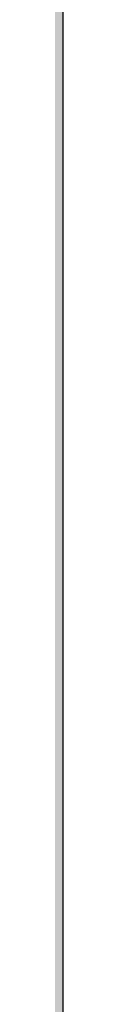
# Model space of a CAD drawing. Units: inches. Extents: x 2091 to 2899, y 967 to 2217.
# Tile 63 of 256: x 2212.1436 to 2212.1443, y 1100.1654 to 1100.4988. Entities that reach past the tile are written whole.
import ezdxf

# ---------------------------------------------------------------- set-up
doc = ezdxf.new("R2010")
doc.units = ezdxf.units.IN
doc.layers.add('A-ANNO-DIMS', color=2, linetype='Continuous', lineweight=18)
doc.layers.add('A-WALL-PATT', color=141, linetype='Continuous', lineweight=13, true_color=0xadddf7)
doc.styles.get("Standard").update_dxf_attribs({"font": 'arial.ttf'})
doc.dimstyles.new('ISO-25', dxfattribs={"dimtxt": 4, "dimasz": 4, "dimexe": 1.25, "dimexo": 0.625, "dimtad": 1, "dimdec": 0, "dimlunit": 3, "dimtxsty": 'Standard', "dimcen": 2.5, "dimadec": 0, "dimazin": 0, "dimtfac": 1, "dimtdec": 0, "dimtmove": 0, "dimatfit": 3, "dimfxl": 1, "dimarcsym": 0})

# ---------------------------------------------------------------- blocks, each defined once
blk = doc.blocks.new('*D71')
at = {"layer": 'A-ANNO-DIMS', "color": 0, "lineweight": -2, "transparency": 16777216}
for p, q in [((2212.1436, 1351.29406), (2212.1436, 969.4643)), ((2452.1436, 1351.29406), (2452.1436, 969.4643)), ((2216.1436, 970.7143), (2448.1436, 970.7143))]:
    blk.add_line(p, q, dxfattribs=at)
at = {"layer": 'A-ANNO-DIMS', "color": 0, "transparency": 16777216}
for points in [[(2216.1436, 971.38097), (2216.1436, 970.04764), (2212.1436, 970.7143)], [(2448.1436, 971.38097), (2448.1436, 970.04764), (2452.1436, 970.7143)]]:
    blk.add_solid(points, dxfattribs=at)
at = {"layer": 'Defpoints', "color": 0, "transparency": 16777216}
for p in [(2212.1436, 1351.91906), (2452.1436, 1351.91906), (2452.1436, 970.7143)]:
    blk.add_point(p, dxfattribs=at)
at = {"layer": 'A-ANNO-DIMS', "color": 0, "transparency": 16777216, "insert": (2332.1436, 973.38159), "char_height": 4, "attachment_point": 5}
blk.add_mtext('20\'-0"', dxfattribs=at)
blk = doc.blocks.new('*D75')
at = {"layer": 'A-ANNO-DIMS', "color": 0, "lineweight": -2, "transparency": 16777216}
for p, q in [((2212.1436, 1274.79406), (2212.1436, 969.4643)), ((2308.1436, 1274.79406), (2308.1436, 969.4643)), ((2216.1436, 970.7143), (2304.1436, 970.7143))]:
    blk.add_line(p, q, dxfattribs=at)
at = {"layer": 'A-ANNO-DIMS', "color": 0, "transparency": 16777216}
for points in [[(2216.1436, 971.38097), (2216.1436, 970.04764), (2212.1436, 970.7143)], [(2304.1436, 971.38097), (2304.1436, 970.04764), (2308.1436, 970.7143)]]:
    blk.add_solid(points, dxfattribs=at)
at = {"layer": 'Defpoints', "color": 0, "transparency": 16777216}
for p in [(2212.1436, 1275.41906), (2308.1436, 1275.41906), (2308.1436, 970.7143)]:
    blk.add_point(p, dxfattribs=at)
at = {"layer": 'A-ANNO-DIMS', "color": 0, "transparency": 16777216, "insert": (2260.1436, 973.38159), "char_height": 4, "attachment_point": 5}
blk.add_mtext('8\'-0"', dxfattribs=at)
blk = doc.blocks.new('*D91')
at = {"layer": 'A-ANNO-DIMS', "color": 0, "lineweight": -2, "transparency": 16777216}
for p, q in [((2211.65063, 1152.24706), (2098.31133, 1152.24706)), ((2099.56133, 1103.91906), (2099.56133, 1148.24706)), ((2211.5186, 1099.91906), (2098.31133, 1099.91906))]:
    blk.add_line(p, q, dxfattribs=at)
at = {"layer": 'A-ANNO-DIMS', "color": 0, "transparency": 16777216}
for points in [[(2098.89467, 1148.24706), (2100.228, 1148.24706), (2099.56133, 1152.24706)], [(2098.89467, 1103.91906), (2100.228, 1103.91906), (2099.56133, 1099.91906)]]:
    blk.add_solid(points, dxfattribs=at)
at = {"layer": 'Defpoints', "color": 0, "transparency": 16777216}
for p in [(2099.56133, 1152.24706), (2212.27563, 1152.24706), (2212.1436, 1099.91906)]:
    blk.add_point(p, dxfattribs=at)
at = {"layer": 'A-ANNO-DIMS', "color": 0, "transparency": 16777216, "insert": (2096.86812, 1126.08306), "char_height": 4, "attachment_point": 5, "rotation": 90}
blk.add_mtext('4\'-4 1/2"', dxfattribs=at)

msp = doc.modelspace()

# ---------------------------------------------------------------- hatches: boundary and pattern name
at = {"layer": 'A-WALL-PATT'}
h = msp.add_hatch(color=256, dxfattribs=at)
h.dxf.hatch_style = 1
h.paths.add_polyline_path([(2803.1436, 2050.91906), (2203.1436, 2050.91906), (2203.1436, 1090.91906), (2803.1436, 1090.91906)])
h.paths.add_polyline_path([(2635.79885, 1147.54046), (2674.52405, 1147.54046, 0.376086), (2678.52967, 1152.8802), (2678.52967, 1159.55647, 0.333335), (2674.52432, 1163.56185), (2674.52432, 1163.56185), (2674.52432, 1192.93439), (2635.80597, 1192.93439), (2597.08762, 1192.93439), (2597.08762, 1163.56185, 0.333335), (2593.08228, 1159.55647), (2593.08228, 1152.8802, 0.376086), (2597.08789, 1147.54046)], flags=0)
h.paths.add_polyline_path([(2436.01043, 1278.24078, 0.000483), (2435.95264, 1278.21503, -0.001328), (2435.93563, 1278.11169, -0.001711), (2436.11644, 1278.04076, 0.002185)], flags=0)
h.paths.add_polyline_path([(2794.1436, 1143.41906), (2794.1436, 1347.41906), (2543.37017, 1347.41906), (2543.37017, 1351.91906), (2794.1436, 1351.91906), (2794.1436, 1392.71355), (2793.9474, 1392.71355), (2793.9474, 1473.5369), (2794.1436, 1473.5369), (2794.1436, 1531.91906), (2650.1436, 1531.91906), (2650.1436, 1536.41906), (2794.1436, 1536.41906), (2794.1436, 1692.41906), (2609.37561, 1692.41906), (2609.37561, 1644.41906), (2604.87561, 1644.41906), (2604.87561, 1744.91906), (2609.37561, 1744.91906), (2609.37561, 1696.91906), (2794.1436, 1696.91906), (2794.1436, 1780.91906), (2609.6436, 1780.91906), (2493.87561, 1780.91906), (2493.87561, 1785.41906), (2609.6436, 1785.41906), (2794.1436, 1785.41906), (2794.1436, 1847.93882), (2793.95122, 1847.93882), (2793.95122, 1928.76217), (2794.1436, 1928.76217), (2794.1436, 1941.41906), (2614.1436, 1941.41906), (2614.1436, 1821.41906), (2609.6436, 1821.41906), (2609.6436, 1941.41906), (2392.1436, 1941.41906), (2392.1436, 1819.91906), (2387.6436, 1819.91906), (2387.6436, 1941.41906), (2212.1436, 1941.41906), (2212.1436, 1783.91906), (2392.1436, 1783.91906), (2392.1436, 1780.91906), (2212.1436, 1780.91906), (2212.1436, 1629.41906), (2387.6436, 1629.41906), (2387.6436, 1744.91906), (2392.1436, 1744.91906), (2392.1436, 1627.91906), (2317.1436, 1627.91906), (2317.1436, 1551.41906), (2317.1436, 1536.41906), (2459.38359, 1536.41906), (2459.38359, 1602.39648), (2463.88359, 1602.39648), (2463.88359, 1531.91906), (2456.6436, 1531.91906), (2456.6436, 1529.91906), (2452.1436, 1529.91906), (2452.1436, 1531.91906), (2312.6436, 1531.91906), (2312.6436, 1551.41906), (2306.1436, 1551.41906), (2306.1436, 1555.91906), (2308.1436, 1555.91906), (2308.1436, 1551.41906), (2312.6436, 1551.41906), (2312.6436, 1627.91906), (2212.1436, 1627.91906), (2212.1436, 1555.91906), (2270.1436, 1555.91906), (2270.1436, 1551.41906), (2212.1436, 1551.41906), (2212.1436, 1351.91906), (2272.1436, 1351.91906), (2272.1436, 1347.41906), (2212.1436, 1347.41906), (2212.1436, 1275.41906), (2308.1436, 1275.41906), (2308.1436, 1351.91906), (2452.1436, 1351.91906), (2452.1436, 1493.91906), (2456.6436, 1493.91906), (2456.6436, 1347.41906), (2312.6436, 1347.41906), (2312.6436, 1270.91906), (2212.1436, 1270.91906), (2212.1436, 1099.91906), (2281.23752, 1099.91906), (2282.87104, 1110.9138), (2282.00834, 1116.9966), (2278.55774, 1121.4204), (2268.20564, 1128.0562), (2272.08764, 1128.0562), (2273.81294, 1131.927), (2279.42034, 1134.6919), (2285.02784, 1135.2449), (2287.61584, 1137.4568), (2288.04714, 1138.0098), (2289.34114, 1140.7747), (2291.06654, 1139.6687), (2292.36054, 1135.2449), (2295.37984, 1136.9038), (2296.24254, 1135.7979), (2297.10524, 1133.033), (2300.12464, 1138.0098), (2303.14394, 1138.0098), (2304.43794, 1135.7979), (2303.14394, 1133.586), (2306.59464, 1134.6919), (2307.88874, 1133.033), (2310.90804, 1135.2449), (2313.92744, 1134.1389), (2315.62686, 1132.4271), (2308.32004, 1117.5496), (2290.20384, 1109.8079), (2288.90984, 1103.1721), (2289.27231, 1099.91906), (2434.91823, 1099.91906), (2431.59323, 1124.78806), (2429.93023, 1169.55306), (2430.92718, 1240.51969), (2435.65893, 1238.18613), (2437.13523, 1196.55406), (2438.79823, 1143.97306), (2442.67823, 1111.99806), (2446.55823, 1099.91906), (2794.1436, 1099.91906), (2794.1436, 1138.91906), (2548.03245, 1138.91906), (2548.03245, 1143.41906), (2548.03245, 1148.81906), (2546.66846, 1148.03156), (2528.68569, 1179.17862, 0.256256), (2512.03245, 1148.81906), (2512.03245, 1143.41906), (2512.03245, 1138.91906), (2507.53245, 1138.91906), (2507.53245, 1143.41906), (2507.53245, 1148.81906, 0.256256), (2490.8792, 1179.17862), (2472.89644, 1148.03156), (2471.53245, 1148.81906), (2471.53245, 1143.41906), (2467.03245, 1143.41906), (2467.03245, 1269.94579, 0.039061), (2460.90999, 1273.58006), (2467.03245, 1273.58006), (2467.03245, 1286.32536, 0.014511), (2465.21619, 1286.76191), (2467.03245, 1287.05258), (2467.03245, 1323.41906), (2471.53245, 1323.41906), (2471.53245, 1148.81906), (2489.53245, 1179.99597), (2490.89644, 1179.20847), (2490.8792, 1179.17862, -0.256256), (2507.53245, 1148.81906), (2507.53245, 1143.41906), (2512.03245, 1143.41906), (2512.03245, 1148.81906, -0.256256), (2528.68569, 1179.17862), (2528.66846, 1179.20847), (2530.03245, 1179.99597), (2548.03245, 1148.81906), (2548.03245, 1143.41906)], flags=16)
h.paths.add_polyline_path([(2607.76855, 1200.94508), (2607.76855, 1265.03063), (2597.08762, 1281.05201), (2619.78459, 1281.05201), (2627.79528, 1337.12686), (2635.79885, 1337.12686), (2643.81666, 1337.12686), (2651.82736, 1281.05201), (2674.52432, 1281.05201), (2663.8434, 1265.03063), (2663.8434, 1200.94508), (2635.80597, 1200.94508)], flags=0)
edge = h.paths.add_edge_path(flags=0)
edge.add_ellipse((13303.89622, 1272.99872), major_axis=(-10595.31304, 0), ratio=0.84230387009, start_angle=0.628237219, end_angle=0.6465541, ccw=False)
edge.add_ellipse((2711.70045, 1156.85268), major_axis=(2.21977, 0), ratio=0.8423039, start_angle=111.53524, end_angle=180.62824, ccw=False)
edge.add_ellipse((13303.15629, 1272.99872), major_axis=(-10593.02631, 0), ratio=0.84230386954, start_angle=0.528271472, end_angle=0.646554097, ccw=False)
edge.add_line((2710.7646, 1175.3333), (2710.12999, 1175.3333))
edge.add_ellipse((2710.12999, 1176.57978), major_axis=(1.47985, 0), ratio=0.8423039, start_angle=180, end_angle=270, ccw=False)
edge.add_line((2708.65014, 1176.57978), (2708.65014, 1200.78291))
edge.add_ellipse((2710.12999, 1200.78291), major_axis=(1.47985, 0), ratio=0.8423039, start_angle=90, end_angle=180, ccw=False)
edge.add_line((2710.12999, 1202.02939), (2710.46508, 1202.02939))
edge.add_ellipse((13303.15629, 1272.99872), major_axis=(-10593.02631, 0), ratio=0.84230386954, start_angle=-0.090229089, end_angle=0.383866779, ccw=False)
edge.add_ellipse((2710.12999, 1290.92703), major_axis=(-1.47985, 0), ratio=0.8423039, start_angle=0, end_angle=90, ccw=False)
edge.add_line((2708.65014, 1290.92703), (2708.65014, 1315.13017))
edge.add_ellipse((2710.12999, 1315.13017), major_axis=(-1.47985, 0), ratio=0.8423039, start_angle=-90, end_angle=0, ccw=False)
edge.add_line((2710.12999, 1316.37665), (2710.70631, 1316.37665))
edge.add_ellipse((3238.40172, 1296.28957), major_axis=(528.234, 0), ratio=0.84230387, start_angle=176.3495724, end_angle=177.8200497, ccw=False)
edge.add_ellipse((2775.06304, 1071.4507), major_axis=(313.30776, 0), ratio=0.84230387, start_angle=102.1259656, end_angle=103.780529, ccw=False)
edge.add_ellipse((2775.06304, 1078.3057), major_axis=(-305.30289, 0), ratio=0.84230387, start_angle=-79.790461, end_angle=-77.5553727, ccw=False)
edge.add_ellipse((2695.14177, 1541.97538), major_axis=(-250.96022, 0), ratio=0.84230387, start_angle=99.256566, end_angle=102.5549326)
edge.add_line((2741.41033, 1334.21426), (2747.13255, 1337.37848))
edge.add_ellipse((2747.53862, 1336.85748), major_axis=(-0.73992, 0), ratio=0.842304, start_angle=270, end_angle=307.93313, ccw=False)
edge.add_ellipse((2747.53862, 1336.85748), major_axis=(-0.73992, 0), ratio=0.842304, start_angle=232.06687, end_angle=270, ccw=False)
edge.add_line((2747.94469, 1337.37848), (2753.66691, 1334.21426))
edge.add_ellipse((2799.93547, 1541.97538), major_axis=(250.96022, 0), ratio=0.84230387, start_angle=257.4450674, end_angle=260.743434)
edge.add_ellipse((2720.01419, 1078.3057), major_axis=(305.30289, 0), ratio=0.84230387, start_angle=77.5553727, end_angle=79.790461, ccw=False)
edge.add_ellipse((2720.01419, 1071.4507), major_axis=(-313.30776, 0), ratio=0.84230387, start_angle=256.219471, end_angle=257.8740344, ccw=False)
edge.add_ellipse((2256.67551, 1296.28957), major_axis=(-528.234, 0), ratio=0.84230387, start_angle=182.1799503, end_angle=183.6504276, ccw=False)
edge.add_line((2784.37092, 1316.37665), (2784.94725, 1316.37665))
edge.add_ellipse((2784.94725, 1315.13017), major_axis=(1.47985, 0), ratio=0.8423039, start_angle=0, end_angle=90, ccw=False)
edge.add_line((2786.42709, 1315.13017), (2786.42709, 1290.92703))
edge.add_ellipse((2784.94725, 1290.92703), major_axis=(1.47985, 0), ratio=0.8423039, start_angle=270, end_angle=360, ccw=False)
edge.add_ellipse((-7808.07906, 1272.99872), major_axis=(10593.02631, 0), ratio=0.84230386954, start_angle=-0.383866779, end_angle=0.090229089, ccw=False)
edge.add_line((2784.61216, 1202.02939), (2784.94725, 1202.02939))
edge.add_ellipse((2784.94725, 1200.78291), major_axis=(1.47985, 0), ratio=0.8423039, start_angle=0, end_angle=90, ccw=False)
edge.add_line((2786.42709, 1200.78291), (2786.42709, 1176.57978))
edge.add_ellipse((2784.94725, 1176.57978), major_axis=(-1.47985, 0), ratio=0.8423039, start_angle=90, end_angle=180, ccw=False)
edge.add_line((2784.94725, 1175.3333), (2784.31264, 1175.3333))
edge.add_ellipse((-7808.07906, 1272.99872), major_axis=(10593.02631, 0), ratio=0.84230386954, start_angle=-0.618643196, end_angle=-0.528271472, ccw=False)
edge.add_ellipse((2783.37678, 1156.85268), major_axis=(-2.21977, 0), ratio=0.8423039, start_angle=179.37176, end_angle=248.46476, ccw=False)
edge.add_ellipse((-7808.81898, 1272.99872), major_axis=(-10595.31304, 0), ratio=0.84230386576, start_angle=179.353445923, end_angle=179.371762803, ccw=False)
edge.add_ellipse((2780.2973, 1153.50079), major_axis=(-5.24643, 0), ratio=0.8423039, start_angle=90, end_angle=179.35345, ccw=False)
edge.add_line((2780.2973, 1149.08171), (2714.77993, 1149.08171))
edge.add_ellipse((2714.77993, 1153.50079), major_axis=(5.24643, 0), ratio=0.8423039, start_angle=180.64655, end_angle=270, ccw=False)
edge = h.paths.add_edge_path(flags=0)
edge.add_line((2718.18737, 1151.00783), (2718.18737, 1170.47236))
edge.add_ellipse((2721.14706, 1170.47236), major_axis=(-2.95969, 0), ratio=0.8423039, start_angle=-90, end_angle=0, ccw=False)
edge.add_line((2721.14706, 1172.96532), (2773.93017, 1172.96532))
edge.add_ellipse((2773.93017, 1170.47236), major_axis=(-2.95969, 0), ratio=0.8423039, start_angle=180, end_angle=270, ccw=False)
edge.add_line((2776.88987, 1170.47236), (2776.88987, 1151.00783))
edge.add_line((2776.88987, 1151.00783), (2718.18737, 1151.00783))
edge = h.paths.add_edge_path(flags=0)
edge.add_line((2718.18737, 1180.23415), (2718.18737, 1199.05783))
edge.add_ellipse((2747.53862, 1320.39864), major_axis=(147.01792, 0), ratio=0.84230387, start_angle=256.4018653, end_angle=283.5981347)
edge.add_line((2776.88987, 1199.05783), (2776.88987, 1180.23415))
edge.add_ellipse((2747.53862, 1301.57496), major_axis=(147.01792, 0), ratio=0.84230387, start_angle=256.4018653, end_angle=283.5981347, ccw=False)
edge = h.paths.add_edge_path(flags=0)
edge.add_ellipse((13303.15629, 1272.99872), major_axis=(-10591.54646, 0), ratio=0.84230386955, start_angle=0.055594314, end_angle=0.377764194, ccw=False)
edge.add_line((2711.61686, 1262.72171), (2715.66741, 1249.4954))
edge.add_ellipse((6413.89196, 1241.69192), major_axis=(-3698.23616, 0), ratio=0.8423038695, start_angle=-0.12089737, end_angle=0.36407635)
edge.add_line((2715.76104, 1218.19245), (2711.93431, 1203.16736))
edge = h.paths.add_edge_path(flags=0)
edge.add_line((2718.18737, 1251.07457), (2716.00249, 1267.45044))
edge.add_ellipse((2742.15117, 1202.18954), major_axis=(81.77258, 0), ratio=0.84230387, start_angle=94.277421, end_angle=111.8349538, ccw=False)
edge.add_line((2737.00975, 1270.93063), (2758.06748, 1270.93063))
edge.add_ellipse((2752.92606, 1202.18954), major_axis=(81.77258, 0), ratio=0.84230387, start_angle=68.1650462, end_angle=85.722579, ccw=False)
edge.add_line((2779.07475, 1267.45044), (2776.88987, 1251.07457))
edge.add_ellipse((2750.33806, 1187.88536), major_axis=(79.57966, 0), ratio=0.84230387, start_angle=67.2080851, end_angle=85.1299304)
edge.add_line((2756.03466, 1254.74366), (2739.04258, 1254.74366))
edge.add_ellipse((2744.73917, 1187.88536), major_axis=(79.57966, 0), ratio=0.84230387, start_angle=94.8700696, end_angle=112.7919149)
edge = h.paths.add_edge_path(flags=0)
edge.add_line((2783.14293, 1203.16736), (2779.31619, 1218.19245))
edge.add_ellipse((-918.81473, 1241.69192), major_axis=(3698.23616, 0), ratio=0.8423038695, start_angle=-0.36407635, end_angle=0.12089737)
edge.add_line((2779.40983, 1249.4954), (2783.46037, 1262.72171))
edge.add_ellipse((-7808.07906, 1272.99872), major_axis=(-10591.54646, 0), ratio=0.84230386954, start_angle=179.622235806, end_angle=179.944405687, ccw=False)
edge = h.paths.add_edge_path(flags=0)
edge.add_ellipse((2734.20089, 1286.69044), major_axis=(-0.35661, 6.34008), ratio=0.6038336, start_angle=89.002014, end_angle=253.657408, ccw=False)
edge.add_line((2730.369, 1286.54181), (2730.369, 1301.35198))
edge.add_line((2730.369, 1301.35198), (2735.91331, 1305.2148))
edge.add_ellipse((2736.38492, 1304.73456), major_axis=(0.73992, 0), ratio=0.842304, start_angle=90, end_angle=134.48021, ccw=False)
edge.add_line((2736.38492, 1305.3578), (2738.03278, 1305.3578))
edge.add_line((2738.03278, 1305.3578), (2738.03278, 1307.70793))
edge.add_ellipse((2794.20164, 1307.70793), major_axis=(56.16886, 0), ratio=0.84230387, start_angle=150.56143, end_angle=180, ccw=False)
edge.add_ellipse((2700.87559, 1307.70793), major_axis=(-56.16886, 0), ratio=0.84230387, start_angle=180, end_angle=209.43857, ccw=False)
edge.add_line((2757.04445, 1307.70793), (2757.04445, 1305.3578))
edge.add_line((2757.04445, 1305.3578), (2758.69232, 1305.3578))
edge.add_ellipse((2758.69232, 1304.73456), major_axis=(-0.73992, 0), ratio=0.842304, start_angle=225.51979, end_angle=270, ccw=False)
edge.add_line((2759.16392, 1305.2148), (2764.70823, 1301.35198))
edge.add_line((2764.70823, 1301.35198), (2764.70823, 1286.54181))
edge.add_ellipse((2760.87634, 1286.69044), major_axis=(0.35661, 6.34008), ratio=0.6038336, start_angle=106.342592, end_angle=270.997986, ccw=False)
edge.add_line((2757.04445, 1285.79709), (2757.04445, 1307.70793))
edge.add_ellipse((2700.87559, 1307.70793), major_axis=(-56.16886, 0), ratio=0.84230387, start_angle=180, end_angle=209.43857)
edge.add_ellipse((2794.20164, 1307.70793), major_axis=(56.16886, 0), ratio=0.84230387, start_angle=150.56143, end_angle=180)
edge.add_line((2738.03278, 1307.70793), (2738.03278, 1285.79709))
h.paths.add_polyline_path([(2417.81227, 1104.4497), (2413.49227, 1102.5297), (2410.61227, 1103.9697), (2409.17227, 1106.3697), (2407.25227, 1107.3297), (2406.29227, 1109.7297), (2405.33227, 1114.0497), (2405.33227, 1117.8897), (2406.29227, 1120.1297), (2407.25227, 1119.8097), (2408.84832, 1118.32766), (2410.17395, 1119.42417), (2410.21127, 1120.4057), (2411.04073, 1121.41905), (2410.69927, 1119.8587), (2410.17395, 1119.42417), (2410.08845, 1117.17611), (2411.13284, 1116.20632), (2413.97227, 1119.3297), (2416.85227, 1120.7697), (2416.86972, 1120.79878), (2417.03507, 1119.40512), (2417.89621, 1118.14338), (2418.29227, 1118.3697), (2419.54445, 1120.03927), (2419.36092, 1118.38749), (2419.03211, 1119.35615), (2418.39894, 1118.51193), (2419.25227, 1114.5297), (2418.79409, 1107.19879)], flags=0)
h.paths.add_polyline_path([(2508.87017, 1347.41906), (2508.37017, 1347.41906), (2508.37017, 1351.91906), (2508.87017, 1351.91906)], flags=0)
h.paths.add_polyline_path([(2473.37017, 1347.41906), (2472.37017, 1347.41906), (2467.87017, 1347.41906), (2467.87017, 1455.41906), (2472.37017, 1455.41906), (2472.37017, 1352.41906), (2473.37017, 1352.41906)], flags=0)
h.paths.add_polyline_path([(2352.10624, 1217.4462), (2349.22624, 1218.8862), (2347.78624, 1221.2862), (2345.86624, 1222.2462), (2344.90624, 1224.6462), (2343.94624, 1228.9662), (2343.94624, 1232.8062), (2344.90624, 1235.0462), (2345.86624, 1234.7262), (2347.46229, 1233.24415), (2348.78792, 1234.34066), (2348.82524, 1235.3222), (2349.6547, 1236.33555), (2349.31324, 1234.7752), (2348.78792, 1234.34066), (2348.70242, 1232.0926), (2349.74681, 1231.12282), (2352.58624, 1234.2462), (2355.46624, 1235.6862), (2355.48369, 1235.71528), (2355.64904, 1234.32161), (2356.51018, 1233.05988), (2356.90624, 1233.2862), (2358.15842, 1234.95576), (2357.97489, 1233.30398), (2357.64608, 1234.27264), (2357.01291, 1233.42842), (2357.86624, 1229.4462), (2357.40806, 1222.11529), (2356.42624, 1219.3662)], flags=0)
h.paths.add_polyline_path([(2348.2968, 1112.22442), (2347.0138, 1112.31042), (2345.5298, 1114.12742), (2345.7318, 1115.85842), (2346.8118, 1116.98242), (2346.8118, 1114.64642), (2345.8668, 1114.21442), (2346.8798, 1114.30042)], flags=0)
h.paths.add_polyline_path([(2347.0138, 1110.92642), (2346.2718, 1110.49342), (2346.6098, 1111.18642)], flags=0)
h.paths.add_polyline_path([(2345.8668, 1118.19442), (2345.5298, 1117.32942), (2343.7078, 1118.02142), (2344.3828, 1118.62642)], flags=0)
h.paths.add_polyline_path([(2346.6768, 1109.28242), (2346.0698, 1108.07142), (2345.8668, 1110.06142)], flags=0)
h.paths.add_polyline_path([(2345.0568, 1119.75142), (2343.6398, 1119.75142), (2343.9778, 1121.13542)], flags=0)
h.paths.add_polyline_path([(2345.2598, 1116.55042), (2345.1248, 1115.85842), (2344.9218, 1115.68542), (2344.7198, 1116.37742)], flags=0)
h.paths.add_polyline_path([(2345.6648, 1112.31042), (2345.4618, 1111.53242), (2344.0448, 1111.96442), (2344.6518, 1112.57042)], flags=0)
h.paths.add_polyline_path([(2345.1918, 1113.34942), (2344.4498, 1113.86842), (2344.7198, 1114.38742)], flags=0)
h.paths.add_polyline_path([(2344.6518, 1116.80942), (2344.1798, 1115.68542), (2344.6518, 1115.33942), (2343.9098, 1114.90642), (2343.0328, 1115.94442), (2343.6398, 1116.46342)], flags=0)
h.paths.add_polyline_path([(2345.8668, 1106.68642), (2344.9898, 1105.56242), (2344.5168, 1106.60042)], flags=0)
h.paths.add_polyline_path([(2344.8548, 1110.06142), (2344.5168, 1109.28242), (2344.1128, 1109.71542)], flags=0)
h.paths.add_polyline_path([(2344.0448, 1113.52242), (2343.4378, 1113.08942), (2342.7628, 1113.95442)], flags=0)
h.paths.add_polyline_path([(2344.3148, 1111.01242), (2342.9648, 1110.32042), (2342.9648, 1111.09942)], flags=0)
h.paths.add_polyline_path([(2345.1248, 1104.69742), (2344.5848, 1103.74542), (2344.4498, 1104.26442)], flags=0)
h.paths.add_polyline_path([(2342.8298, 1121.22242), (2341.7498, 1120.53042), (2340.5358, 1121.04942), (2340.1308, 1121.82842), (2340.6708, 1122.95242), (2341.1428, 1121.82842), (2341.6148, 1122.00142)], flags=0)
h.paths.add_polyline_path([(2342.9648, 1119.75142), (2343.0328, 1118.45342), (2342.0878, 1118.02142), (2342.0198, 1119.49142)], flags=0)
h.paths.add_polyline_path([(2342.6948, 1116.89642), (2341.9528, 1116.63642), (2342.0198, 1117.32942)], flags=0)
h.paths.add_polyline_path([(2343.0328, 1112.22442), (2342.0198, 1111.79142), (2341.5478, 1112.22442), (2342.3578, 1113.34942)], flags=0)
h.paths.add_polyline_path([(2343.7748, 1104.43742), (2342.6278, 1102.88042), (2342.6948, 1104.61042), (2343.4378, 1105.12942)], flags=0)
h.paths.add_polyline_path([(2342.0198, 1115.07942), (2340.8058, 1115.51242), (2340.9408, 1116.37742)], flags=0)
h.paths.add_polyline_path([(2341.4808, 1120.09742), (2341.4808, 1119.40542), (2341.0758, 1119.57842), (2341.1428, 1120.09742)], flags=0)
h.paths.add_polyline_path([(2341.8178, 1114.47342), (2340.9408, 1113.08942), (2340.8058, 1114.56042)], flags=0)
h.paths.add_polyline_path([(2341.1428, 1118.54042), (2340.9408, 1116.98242), (2339.0508, 1117.67542), (2339.0508, 1118.62642)], flags=0)
h.paths.add_polyline_path([(2342.6948, 1101.66842), (2341.9528, 1101.84142), (2342.5598, 1102.36142)], flags=0)
h.paths.add_polyline_path([(2340.3328, 1119.66542), (2338.4438, 1119.57842), (2337.9038, 1120.35742), (2339.6578, 1120.61642)], flags=0)
h.paths.add_polyline_path([(2340.3328, 1115.33942), (2340.0628, 1113.69542), (2339.3878, 1115.33942)], flags=0)
h.paths.add_polyline_path([(2341.8178, 1103.83142), (2341.5478, 1102.88042), (2341.1428, 1103.65842)], flags=0)
h.paths.add_polyline_path([(2339.0508, 1122.86642), (2337.2958, 1121.82842), (2337.0938, 1123.12542), (2337.7688, 1123.81842)], flags=0)
h.paths.add_polyline_path([(2339.1178, 1121.74142), (2338.8478, 1121.22242), (2338.1738, 1121.04942), (2338.3758, 1121.56842)], flags=0)
h.paths.add_polyline_path([(2339.1858, 1119.31942), (2338.6458, 1118.71342), (2338.2408, 1118.10742), (2338.2408, 1118.88642)], flags=0)
h.paths.add_polyline_path([(2341.1428, 1101.92842), (2340.6028, 1101.23642), (2340.0628, 1101.84142), (2340.6028, 1102.36142)], flags=0)
h.paths.add_polyline_path([(2337.6338, 1117.76142), (2336.6208, 1118.28042), (2337.2958, 1118.97242)], flags=0)
h.paths.add_polyline_path([(2336.8238, 1119.57842), (2334.7988, 1118.97242), (2335.2038, 1120.35742), (2336.5538, 1120.87642)], flags=0)
h.paths.add_polyline_path([(2339.1178, 1100.45742), (2337.3638, 1100.54342), (2336.7558, 1101.23642)], flags=0)
h.paths.add_polyline_path([(2336.3508, 1122.43342), (2336.0138, 1121.91442), (2334.9338, 1122.43342), (2334.5288, 1123.47142), (2335.7438, 1122.77942)], flags=0)
h.paths.add_polyline_path([(2334.7318, 1120.87642), (2334.2588, 1120.35742), (2334.0568, 1120.78942), (2334.5968, 1121.30842)], flags=0)
h.paths.add_polyline_path([(2334.4618, 1122.17442), (2332.5718, 1121.30842), (2331.3568, 1122.17442), (2332.0998, 1122.86642)], flags=0)
h.paths.add_polyline_path([(2334.2588, 1118.54042), (2333.3818, 1118.45342), (2333.6518, 1119.31942)], flags=0)
h.paths.add_polyline_path([(2335.5418, 1102.27442), (2334.1918, 1102.62042), (2335.2718, 1103.31242)], flags=0)
h.paths.add_polyline_path([(2332.7068, 1119.66542), (2331.6948, 1120.44342), (2332.5048, 1120.78942)], flags=0)
h.paths.add_polyline_path([(2334.7318, 1101.14942), (2333.5168, 1101.58242), (2333.9888, 1101.75542)], flags=0)
h.paths.add_polyline_path([(2332.6398, 1116.63642), (2331.0868, 1116.29042), (2331.9648, 1118.19442)], flags=0)
h.paths.add_polyline_path([(2330.7498, 1121.56842), (2330.2768, 1120.27042), (2328.5228, 1119.31942), (2328.9948, 1121.04942)], flags=0)
h.paths.add_polyline_path([(2330.7498, 1118.62642), (2330.0078, 1117.50242), (2329.8728, 1118.02142)], flags=0)
h.paths.add_polyline_path([(2332.0998, 1102.36142), (2330.5468, 1102.01442), (2331.6948, 1102.96642)], flags=0)
h.paths.add_polyline_path([(2329.5348, 1113.60842), (2329.0628, 1112.31042), (2328.5898, 1113.34942)], flags=0)
h.paths.add_polyline_path([(2328.3878, 1117.84842), (2327.5098, 1116.55042), (2327.1728, 1117.76142)], flags=0)
h.paths.add_polyline_path([(2329.7378, 1106.51342), (2329.5348, 1105.30242), (2328.2528, 1106.08142)], flags=0)
h.paths.add_polyline_path([(2328.6578, 1114.38742), (2328.0498, 1114.12742), (2328.3198, 1114.90642)], flags=0)
h.paths.add_polyline_path([(2328.3198, 1112.22442), (2327.1058, 1112.13742), (2326.7008, 1112.65642)], flags=0)
h.paths.add_polyline_path([(2326.9028, 1115.25242), (2326.7008, 1114.12742), (2325.2158, 1113.60842), (2326.0928, 1115.33942)], flags=0)
h.paths.add_polyline_path([(2326.6328, 1108.33042), (2326.0928, 1107.37942), (2325.8908, 1108.50342), (2326.4978, 1109.10942)], flags=0)
h.paths.add_polyline_path([(2615.1436, 1531.91906), (2609.6436, 1531.91906), (2609.6436, 1620.41906), (2614.1436, 1620.41906), (2614.1436, 1536.41906), (2615.1436, 1536.41906)], flags=0)
h.paths.add_polyline_path([(2545.1436, 1563.41906), (2464.1436, 1563.41906), (2464.1436, 1632.41906), (2509.1436, 1632.41906), (2509.1436, 1627.91906), (2509.1436, 1603.91906), (2468.6436, 1603.91906), (2468.6436, 1567.91906), (2540.6436, 1567.91906), (2540.6436, 1591.91906), (2545.1436, 1591.91906)], flags=0)
h.paths.add_polyline_path([(2388.96905, 1549.98573), (2357.43418, 1549.98573), (2357.43418, 1623.36078), (2399.36278, 1623.36078), (2435.68947, 1623.36078), (2435.59255, 1602.55927), (2435.59255, 1602.39648), (2388.96905, 1602.39648)], flags=0)
h.paths.add_polyline_path([(2388.88063, 1555.80915), (2374.90443, 1555.80915), (2374.90443, 1600.57156), (2374.90443, 1615.45765), (2406.35088, 1615.45765), (2406.35088, 1618.93943), (2412.17429, 1615.45765), (2406.35088, 1611.97586), (2406.35088, 1615.45765), (2388.88063, 1615.45765)], flags=0)
h.paths.add_polyline_path([(2568.87561, 1644.41906), (2453.37561, 1644.41906), (2453.37561, 1785.41906), (2457.87561, 1785.41906), (2457.87561, 1648.91906), (2568.87561, 1648.91906)], flags=0)
h.paths.add_polyline_path([(2212.1436, 1945.91906), (2212.1436, 2041.91906), (2794.1436, 2041.91906), (2794.1436, 1945.91906)], flags=16)
h.paths.add_polyline_path([(2271.08273, 1964.31724), (2776.85297, 1964.31724), (2776.85297, 2037.16962), (2271.08273, 2037.16962)], flags=8)
h.paths.add_polyline_path([(2380.64929, 1536.82414), (2461.04081, 1536.82414), (2461.04081, 1554.65259), (2380.64929, 1554.65259)], flags=8)
h.paths.add_polyline_path([(2240.75571, 1609.72545), (2309.18583, 1609.72545), (2309.18583, 1617.6982), (2240.75571, 1617.6982)], flags=8)
h.paths.add_polyline_path([(2212.67726, 1313.5041), (2282.59152, 1313.5041), (2282.59152, 1322.74524), (2212.67726, 1322.74524)], flags=8)
h.paths.add_polyline_path([(2457.11198, 1114.77857), (2558.48158, 1114.77857), (2558.48158, 1142.21968), (2457.11198, 1142.21968)], flags=8)
h.paths.add_polyline_path([(2473.44234, 1273.01007), (2604.64123, 1273.01007), (2604.64123, 1318.34693), (2473.44234, 1318.34693)], flags=8)
h.paths.add_polyline_path([(2638.8763, 1626.97743), (2684.25037, 1627.97674), (2684.03848, 1637.59749), (2638.66442, 1636.59819)], flags=8)
h.paths.add_polyline_path([(2537.59055, 1453.79345), (2628.38955, 1453.79345), (2628.38955, 1475.34481), (2537.59055, 1475.34481)], flags=8)
h.paths.add_polyline_path([(2504.13764, 1714.6324), (2554.64719, 1714.6324), (2554.64719, 1730.23771), (2504.13764, 1730.23771)], flags=8)
h.paths.add_polyline_path([(2487.50118, 1575.65187), (2535.09712, 1575.65187), (2535.09712, 1598.37765), (2487.50118, 1598.37765)], flags=8)
h.paths.add_polyline_path([(2709.0994, 1735.71028), (2740.0166, 1735.71028), (2740.0166, 1749.93764), (2709.0994, 1749.93764)], flags=8)
h.paths.add_polyline_path([(2442.43842, 1792.17166), (2564.72884, 1792.17166), (2564.72884, 1842.00016), (2442.43842, 1842.00016)], flags=8)
h.paths.add_polyline_path([(2655.8158, 1809.64408), (2789.52014, 1806.6938), (2790.08498, 1832.29164), (2656.38064, 1835.24192)], flags=8)
h.paths.add_polyline_path([(2234.8427, 1797.72014), (2368.59285, 1794.76885), (2369.16072, 1820.50413), (2235.41056, 1823.45542)], flags=8)
h.paths.add_polyline_path([(2245.13847, 1644.00633), (2398.42773, 1640.6239), (2398.99484, 1666.32482), (2245.70557, 1669.70725)], flags=8)
h.paths.add_polyline_path([(2306.14285, 1431.16852), (2413.76831, 1428.79369), (2414.33315, 1454.39153), (2306.70768, 1456.76636)], flags=8)
h.paths.add_polyline_path([(2306.83458, 1458.23314), (2393.38048, 1456.32345), (2393.93281, 1481.35436), (2307.38691, 1483.26405)], flags=8)

# ---------------------------------------------------------------- dimensions: what is measured, and where the dimension line sits
at = {"layer": 'A-ANNO-DIMS'}
for base, p1, p2, picture, middle in [((2452.1436, 970.7143), (2212.1436, 1351.91906), (2452.1436, 1351.91906), '*D71', (2332.1436, 973.38159)), ((2308.1436, 970.7143), (2212.1436, 1275.41906), (2308.1436, 1275.41906), '*D75', (2260.1436, 973.38159))]:
    dim = msp.add_linear_dim(base=base, p1=p1, p2=p2, dimstyle='ISO-25', override={"dimdec": 1, "dimlfac": 1, "dimrnd": 0, "dimzin": 1, "dimdsep": 46, "dimlunit": 4, "dimfrac": 2}, dxfattribs=at)
    dim.commit()
    dim.dimension.update_dxf_attribs({"geometry": picture, "text_midpoint": middle})
dim = msp.add_linear_dim(base=(2099.56133, 1152.24706), p1=(2212.1436, 1099.91906), p2=(2212.27563, 1152.24706), angle=90, dimstyle='ISO-25', override={"dimdec": 1, "dimlfac": 1, "dimrnd": 0, "dimzin": 1, "dimdsep": 46, "dimlunit": 4, "dimfrac": 2}, dxfattribs=at)
dim.commit()
dim.dimension.update_dxf_attribs({"geometry": '*D91', "text_midpoint": (2096.86812, 1126.08306)})

doc.saveas('drawing.dxf')
